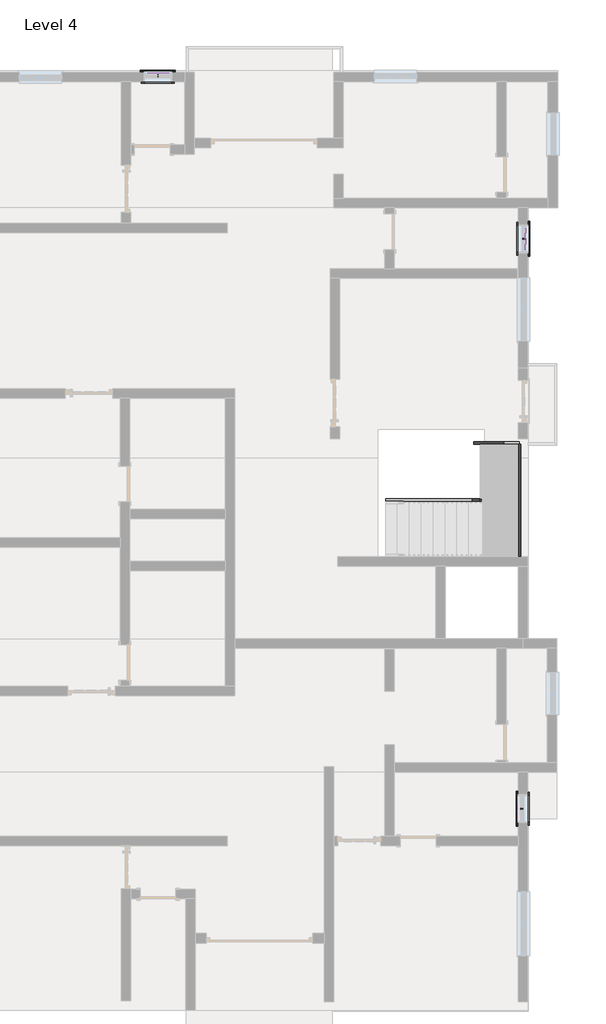
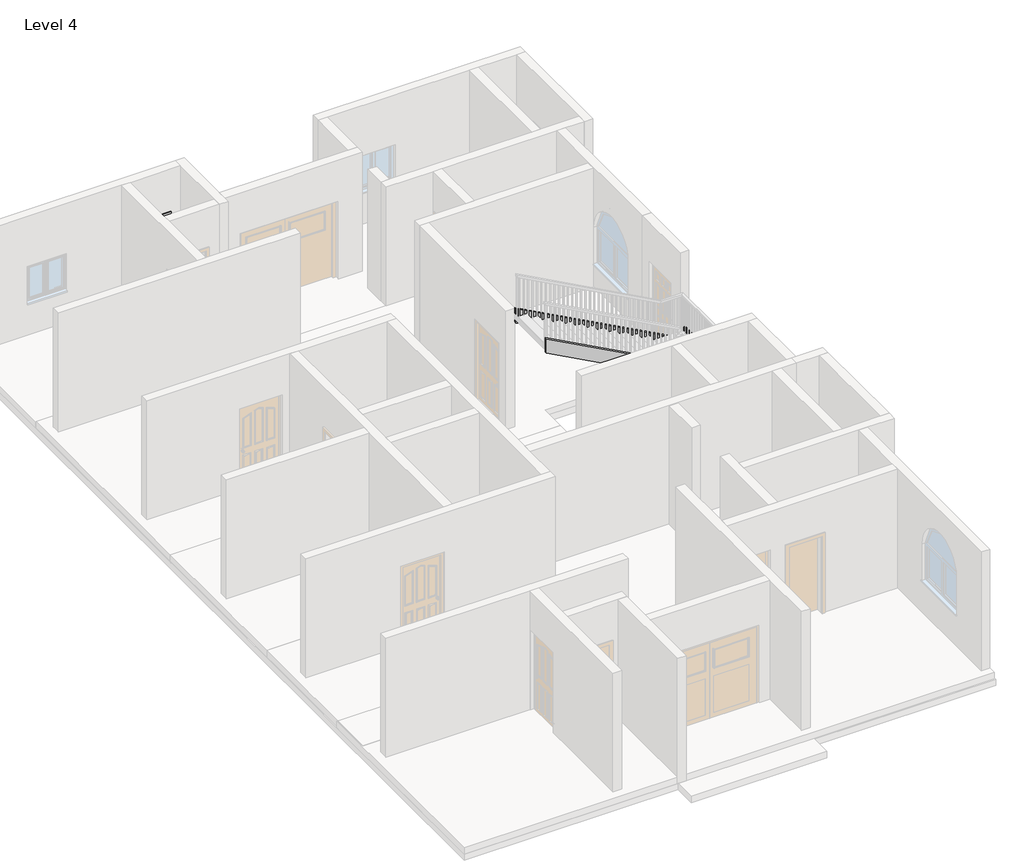
# One storey, part 7 of 7: 11 proxies, 5 members.
"""IFC4 building model written with IfcOpenShell, lengths in millimetres."""

from ifc_helpers import new_model, si_unit, frame, origin, place, context, project, spatial, polyline, outline, extrude, transform, mapped, element, save
from components import muntin_pattern_2x2_muntin_pattern_2x2_eba6c5fb, trim_window_exterior_flat_with_sill_278e6a94, trim_window_interior_flat_picture_frame_e9fd5f45

model = new_model("IFC4")

# Units and contexts
model_context = context("Model", 3, world=origin())
ifc_project = project(units=[si_unit("LENGTHUNIT", "METRE", prefix="MILLI")], contexts=[model_context])

# Site, building, storey
site = spatial("IfcSite", under=ifc_project)
building = spatial("IfcBuilding", under=site)
storey = spatial("IfcBuildingStorey", under=building, Name="Level 4", Elevation=9144.0)

# Proxies
placement = place(None, origin())
muntin_pattern_2x2_muntin_pattern_2x2_shape = muntin_pattern_2x2_muntin_pattern_2x2_eba6c5fb(model_context)
element("IfcBuildingElementProxy", 1, Name="Muntin Pattern_2x2 : Muntin Pattern_2x2", ObjectType="Muntin Pattern_2x2 : Muntin Pattern_2x2", at=placement, inside=storey, context=model_context, shape_type="MappedRepresentation", body=[
    mapped(muntin_pattern_2x2_muntin_pattern_2x2_shape, transform((5828.2640963, 5846.2962251, 10614.025), x_axis=(0.0, -1.0, 0.0), y_axis=(1.0, 0.0, 0.0), z_axis=(0.0, 0.0, 1.0))),
])
element("IfcBuildingElementProxy", 2, Name="Muntin Pattern_2x2 : Muntin Pattern_2x2", ObjectType="Muntin Pattern_2x2 : Muntin Pattern_2x2", at=placement, inside=storey, context=model_context, shape_type="MappedRepresentation", body=[
    mapped(muntin_pattern_2x2_muntin_pattern_2x2_shape, transform((5783.8140963, 5846.2962251, 10134.6), x_axis=(0.0, -1.0, 0.0), y_axis=(1.0, 0.0, 0.0), z_axis=(0.0, 0.0, 1.0))),
])
element("IfcBuildingElementProxy", 3, Name="Muntin Pattern_2x2 : Muntin Pattern_2x2", ObjectType="Muntin Pattern_2x2 : Muntin Pattern_2x2", at=placement, inside=storey, context=model_context, shape_type="MappedRepresentation", body=[
    mapped(muntin_pattern_2x2_muntin_pattern_2x2_shape, transform((5739.3640963, -6313.9537749, 10134.6), x_axis=(0.0, 1.0, 0.0), y_axis=(-1.0, 0.0, 0.0), z_axis=(0.0, 0.0, 1.0))),
])
element("IfcBuildingElementProxy", 4, Name="Muntin Pattern_2x2 : Muntin Pattern_2x2", ObjectType="Muntin Pattern_2x2 : Muntin Pattern_2x2", at=placement, inside=storey, context=model_context, shape_type="MappedRepresentation", body=[
    mapped(muntin_pattern_2x2_muntin_pattern_2x2_shape, transform((-2029.8609037, 9366.9277313, 10614.025), x_axis=(1.0, 0.0, 0.0), y_axis=(0.0, 1.0, 0.0), z_axis=(0.0, 0.0, 1.0))),
])
element("IfcBuildingElementProxy", 5, Name="Muntin Pattern_2x2 : Muntin Pattern_2x2", ObjectType="Muntin Pattern_2x2 : Muntin Pattern_2x2", at=placement, inside=storey, context=model_context, shape_type="MappedRepresentation", body=[
    mapped(muntin_pattern_2x2_muntin_pattern_2x2_shape, transform((-2029.8609037, 9322.4777313, 10134.6), x_axis=(1.0, 0.0, 0.0), y_axis=(0.0, 1.0, 0.0), z_axis=(0.0, 0.0, 1.0))),
])
trim_window_exterior_flat_with_sill_shape = trim_window_exterior_flat_with_sill_278e6a94(model_context)
element("IfcBuildingElementProxy", 6, Name="Trim-Window-Exterior-Flat : with Sill", ObjectType="Trim-Window-Exterior-Flat : with Sill", at=placement, inside=storey, context=model_context, shape_type="MappedRepresentation", body=[
    mapped(trim_window_exterior_flat_with_sill_shape, transform((5863.1890963, 5846.2962251, 11125.2), x_axis=(0.0, 1.0, 0.0), y_axis=(0.0, 0.0, 1.0), z_axis=(1.0, 0.0, 0.0))),
])
element("IfcBuildingElementProxy", 7, Name="Trim-Window-Exterior-Flat : with Sill", ObjectType="Trim-Window-Exterior-Flat : with Sill", at=placement, inside=storey, context=model_context, shape_type="MappedRepresentation", body=[
    mapped(trim_window_exterior_flat_with_sill_shape, transform((5659.9890963, -6313.9537749, 11125.2), x_axis=(0.0, -1.0, 0.0), y_axis=(0.0, 0.0, 1.0), z_axis=(-1.0, 0.0, 0.0))),
])
element("IfcBuildingElementProxy", 8, Name="Trim-Window-Exterior-Flat : with Sill", ObjectType="Trim-Window-Exterior-Flat : with Sill", at=placement, inside=storey, context=model_context, shape_type="MappedRepresentation", body=[
    mapped(trim_window_exterior_flat_with_sill_shape, transform((-2029.8609037, 9401.8527313, 11125.2), x_axis=(-1.0, 0.0, 0.0), y_axis=(0.0, 0.0, 1.0), z_axis=(0.0, 1.0, 0.0))),
])
trim_window_interior_flat_picture_frame_shape = trim_window_interior_flat_picture_frame_e9fd5f45(model_context)
element("IfcBuildingElementProxy", 9, Name="Trim-Window-Interior-Flat : Picture Frame", ObjectType="Trim-Window-Interior-Flat : Picture Frame", at=placement, inside=storey, context=model_context, shape_type="MappedRepresentation", body=[
    mapped(trim_window_interior_flat_picture_frame_shape, transform((5659.9890963, 5846.2962251, 11125.2), x_axis=(0.0, -1.0, 0.0), y_axis=(0.0, 0.0, 1.0), z_axis=(-1.0, 0.0, 0.0))),
])
element("IfcBuildingElementProxy", 10, Name="Trim-Window-Interior-Flat : Picture Frame", ObjectType="Trim-Window-Interior-Flat : Picture Frame", at=placement, inside=storey, context=model_context, shape_type="MappedRepresentation", body=[
    mapped(trim_window_interior_flat_picture_frame_shape, transform((5863.1890963, -6313.9537749, 11125.2), x_axis=(0.0, 1.0, 0.0), y_axis=(0.0, 0.0, 1.0), z_axis=(1.0, 0.0, 0.0))),
])
element("IfcBuildingElementProxy", 11, Name="Trim-Window-Interior-Flat : Picture Frame", ObjectType="Trim-Window-Interior-Flat : Picture Frame", at=placement, inside=storey, context=model_context, shape_type="MappedRepresentation", body=[
    mapped(trim_window_interior_flat_picture_frame_shape, transform((-2029.8609037, 9198.6527313, 11125.2), x_axis=(1.0, 0.0, 0.0), y_axis=(0.0, 0.0, 1.0), z_axis=(0.0, -1.0, 0.0))),
])

# Members
element("IfcMember", 12, ObjectType="Stringer - 2\" Width", at=placement, inside=storey, context=model_context, shape_type="SweptSolid", body=[
    extrude(outline(polyline([(9351.8380635, 2827.8890963), (9144.0, 2827.8890963), (9144.0, 3084.6852277), (10084.9274897, 4830.2326586), (10431.1900583, 4830.2326586), (9351.8380635, 2827.8890963)])), frame((0.0, 245.5962251, 0.0), z_axis=(0.0, 1.0, 0.0), x_axis=(0.0, 0.0, 1.0)), (0.0, 0.0, 1.0), 50.8),
])
element("IfcMember", 13, ObjectType="Stringer - 2\" Width", at=placement, inside=storey, context=model_context, shape_type="SweptSolid", body=[
    extrude(outline(polyline([(10250.7131227, 4881.0326586), (10597.3108372, 4881.0326586), (12258.8157251, 1811.8890963), (11912.2180107, 1811.8890963), (10250.7131227, 4881.0326586)])), frame((0.0, 245.5962251, 0.0), z_axis=(0.0, 1.0, 0.0), x_axis=(0.0, 0.0, 1.0)), (0.0, 0.0, 1.0), 50.8),
])
element("IfcMember", 14, ObjectType="Stringer - 2\" Width", at=placement, inside=storey, context=model_context, shape_type="SweptSolid", body=[
    extrude(outline(polyline([(9351.8380635, 2827.8890963), (9144.0, 2827.8890963), (9144.0, 3084.6852277), (10467.1090909, 5539.2310877), (10467.1090909, 4896.8673098), (9351.8380635, 2827.8890963)])), frame((0.0, -986.3037749, 0.0), z_axis=(0.0, 1.0, 0.0), x_axis=(0.0, 0.0, 1.0)), (0.0, 0.0, 1.0), 50.8),
])
element("IfcMember", 15, ObjectType="Stringer - 2\" Width", at=placement, inside=storey, context=model_context, shape_type="SweptSolid", body=[
    extrude(outline(polyline([(5710.7890963, -986.3037749), (5659.9890963, -986.3037749), (5659.9890963, 1464.7962251), (5710.7890963, 1464.7962251), (5710.7890963, -986.3037749)])), frame((0.0, 0.0, 10162.3090909), z_axis=(0.0, 0.0, 1.0), x_axis=(1.0, 0.0, 0.0)), (0.0, 0.0, 1.0), 304.8),
])
element("IfcMember", 16, ObjectType="Stringer - 2\" Width", at=placement, inside=storey, context=model_context, shape_type="SweptSolid", body=[
    extrude(outline(polyline([(10162.3090909, 5684.5709562), (12258.8157251, 1811.8890963), (11912.2180107, 1811.8890963), (10162.3090909, 5044.3332105), (10162.3090909, 5684.5709562)])), frame((0.0, 1464.7962251, 0.0), z_axis=(0.0, 1.0, 0.0), x_axis=(0.0, 0.0, 1.0)), (0.0, 0.0, 1.0), 50.8),
])

save(model, "model.ifc")

# Revit data of these elements
# Type "Muntin Pattern_2x2 : Muntin Pattern_2x2"
#   Width [instance default] = 4' - 0"
#   Thickness = 0' - 0 1/2"
#   Height [instance default] = 4' - 0"
#   Distance = 0' - 0 3/4"
#   Interior Material [instance default] = none
#   Exterior Material [instance default] = none
#   Default Elevation = 0
# Type "Trim-Window-Exterior-Flat : with Sill"
#   Trim Width = 0' - 2 1/4"
#   Trim Thickness_Picture Frame = 0' - 1 1/4"
#   Trim Thickness_with Sill = 0' - 0 3/4"
#   Sill Thickness = 0' - 1 1/4"
#   Opening Width [instance default] = 2' - 0"
#   Opening Height [instance default] = 3' - 0"
#   Default Elevation = 4' - 0"
#   Sill = yes
#   Picture Frame = no
#   Trim Material [instance default] = none
# Type "Trim-Window-Interior-Flat : Picture Frame"
#   Trim Thickness_Picture Frame = 0' - 1 1/4"
#   Trim Width = 0' - 2 1/4"
#   Trim Thickness_with Sill = 0' - 0 3/4"
#   Sill Thickness = 0' - 1 1/4"
#   Opening Width [instance default] = 2' - 0"
#   Opening Height [instance default] = 3' - 0"
#   Default Elevation = 4' - 0"
#   Sill = no
#   Picture Frame = yes
#   Trim Material [instance default] = none
# Elements 1, 2, 3, 4, 5 (IfcBuildingElementProxy, "Muntin Pattern_2x2 : Muntin Pattern_2x2")
#   Width = 1' - 6"
#   Height = 1' - 5 1/8"
#   Interior Material = Wood - Stained
#   Exterior Material = Clad - White
#   Phase Created = New Construction
#   Materials on its faces: "Clad - White", "Wood - Stained"
# Elements 6, 7, 8 (IfcBuildingElementProxy, "Trim-Window-Exterior-Flat : with Sill")
#   Opening Width = 2' - 0"
#   Opening Height = 3' - 6"
#   Trim Material = Clad - White
#   Phase Created = New Construction
#   Materials on its faces: "Clad - White"
# Elements 9, 10, 11 (IfcBuildingElementProxy, "Trim-Window-Interior-Flat : Picture Frame")
#   Opening Width = 2' - 0"
#   Opening Height = 3' - 6"
#   Trim Material = Wood - Stained
#   Phase Created = New Construction
#   Materials on its faces: "Wood - Stained"
# Elements 12, 13, 14, 15, 16 (IfcMember, "Stringer - 2\" Width")
#   Phase Created = New Construction
# Materials
#   "Clad - White": class "Wood", colour RGB 242 242 238, transparency 0, Cost = 0
#   "Wood - Stained": class "Wood", colour RGB 224 178 126, transparency 0, Cost = 0
